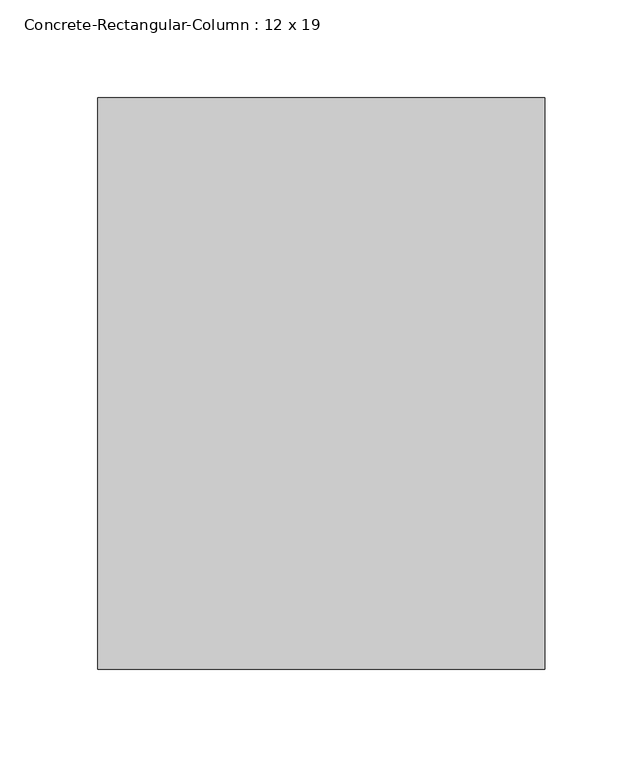
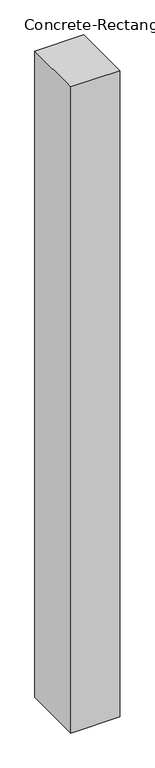
"""IFC4 building model written with IfcOpenShell, lengths in millimetres: column geometry, Concrete-Rectangular-Column : 12 x 19."""

from ifc_helpers import new_model, si_unit, frame, origin, place, context, project, spatial, polyline, outline, extrude, source, transform, mapped, element, save


def concrete_rectangular_column_12_x_19_f479a93c(model_context):
    return source(origin(), model_context, "Body", "SweptSolid", [
        extrude(outline(polyline([(114.3, 146.05), (114.3, -146.05), (-114.3, -146.05), (-114.3, 146.05), (114.3, 146.05)])), frame((0.0, 0.0, 3200.4), z_axis=(0.0, 0.0, 1.0), x_axis=(1.0, 0.0, 0.0)), (0.0, 0.0, 1.0), 3200.4),
    ])


if __name__ == "__main__":
    model = new_model("IFC4")
    model_context = context("Model", 3, world=origin())
    ifc_project = project(units=[si_unit("LENGTHUNIT", "METRE", prefix="MILLI")], contexts=[model_context])
    site = spatial("IfcSite", under=ifc_project)
    building = spatial("IfcBuilding", under=site)
    placement = place(None, origin())
    concrete_rectangular_column_12_x_19_shape = concrete_rectangular_column_12_x_19_f479a93c(model_context)
    element("IfcColumn", 1, ObjectType="Concrete-Rectangular-Column : 12 x 19", at=placement, inside=building, context=model_context, shape_type="MappedRepresentation", body=[
        mapped(concrete_rectangular_column_12_x_19_shape, transform((0.0, 0.0, 0.0), x_axis=(1.0, 0.0, 0.0), y_axis=(0.0, 1.0, 0.0), z_axis=(0.0, 0.0, 1.0))),
    ])
    save(model, "model.ifc")

# Revit data of these elements
# Type "Concrete-Rectangular-Column : 12 x 19"
#   Assembly Code = "B10"
#   b = 0' - 9"
#   h = 0' - 11 1/2"
#   Structural Material [instance default] = Concrete, Cast-in-Place gray
# Element 1 (IfcColumn, "Concrete-Rectangular-Column : 12 x 19")
#   Structural Material = Concrete Masonry Units
#   Materials on its faces: "Concrete Masonry Units"
# Materials
#   "Concrete, Cast-in-Place gray": class "Concrete", colour RGB 192 192 192, transparency 0, Description = "Cast-in-place concrete", Cost = 0
#   "Concrete Masonry Units": class "Masonry", colour RGB 63 63 63, transparency 0, Description = "Concrete masonry units", Cost = 0
